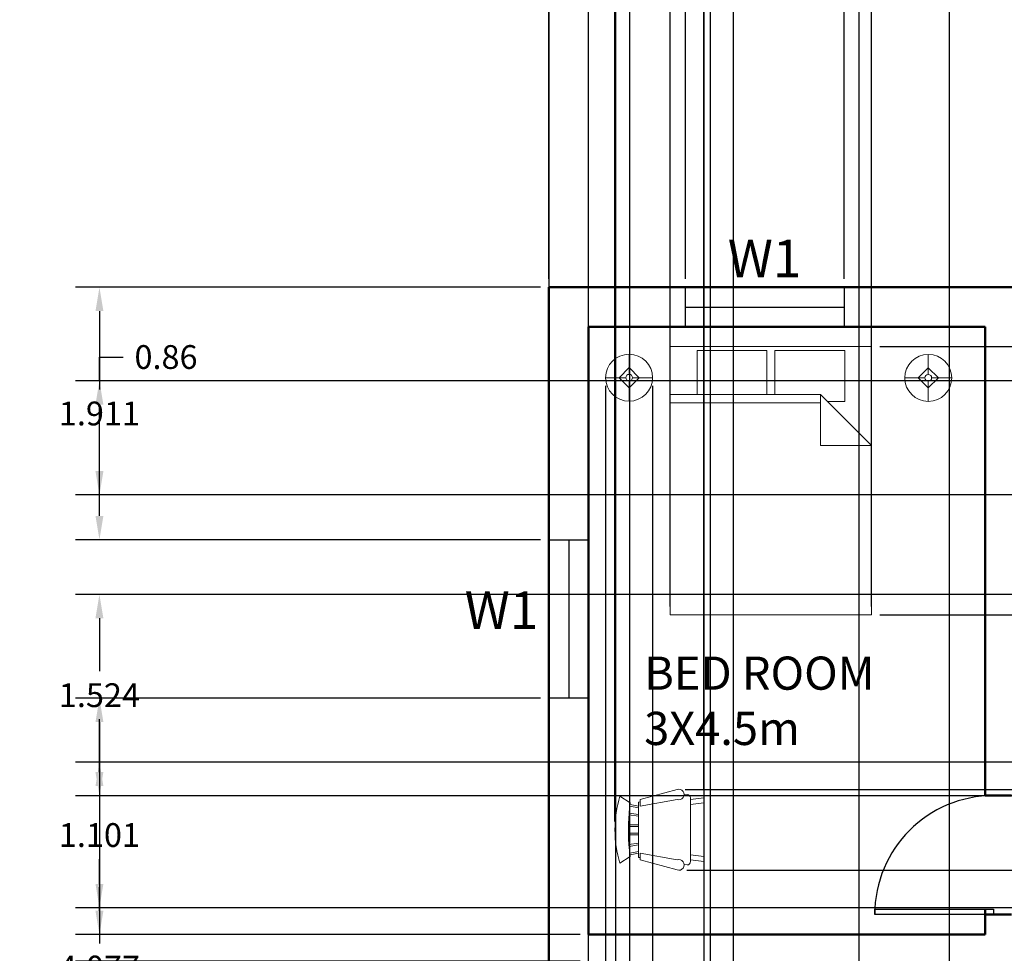
# Model space of a CAD drawing. Units: metres. Extents: x 2443.7 to 2482.9, y 2261.4 to 2287.
# Tile 3 of 8: x 2443.7 to 2451.1, y 2269.7 to 2276.8. Entities that reach past the tile are written whole.
import ezdxf

# ---------------------------------------------------------------- set-up
doc = ezdxf.new("R2010")
doc.units = ezdxf.units.M
for name, color, linetype, lineweight in [('A-ANNO-DIMS', 2, 'Continuous', 18), ('A-AREA-IDEN', 11, 'Continuous', 25), ('A-MODL', 7, 'Continuous', 25), ('A-WALL', 7, 'Continuous', 50), ('door', 6, 'Continuous', 25), ('furnitures', 20, 'Continuous', 18), ('text', 11, 'Continuous', 25), ('window', 3, 'Continuous', 25)]:
    doc.layers.add(name, color=color, linetype=linetype, lineweight=lineweight)
doc.styles.get("Standard").update_dxf_attribs({"font": 'arial.ttf'})
doc.dimstyles.get("Standard").update_dxf_attribs({"dimtxt": 0.18, "dimasz": 0.18, "dimexe": 0.18, "dimexo": 0.0625, "dimgap": 0.09, "dimtad": 0, "dimtih": 1, "dimtoh": 1, "dimdec": 4, "dimzin": 0, "dimdsep": 46, "dimtxsty": 'Standard', "dimcen": 0.09, "dimadec": 0, "dimazin": 0, "dimtfac": 1, "dimtdec": 4, "dimtofl": 0, "dimtmove": 0, "dimatfit": 3, "dimfxl": 1, "dimtolj": 1, "dimtzin": 0, "dimarcsym": 0})

# ---------------------------------------------------------------- blocks, each defined once
blk = doc.blocks.new('*U21')
for p, q in [((0, 0), (0, -6)), ((40, 0), (40, -6))]:
    blk.add_line(p, q)
blk.add_lwpolyline([(0, 0), (0, 40), (1.75, 40), (1.75, 0)], close=True)
blk.add_arc((0, 0), 40, 0, 90)
blk = doc.blocks.new('Bed - Queen')
for p, q in [((0, -80.00003), (0, 0)), ((0, 0), (59.99999, 0)), ((59.99999, 0), (59.99999, -80.00003)), ((7.99999, -1.2), (28.79998, -1.2)), ((7.99999, -14.4), (7.99999, -1.2)), ((28.79998, -1.2), (28.79998, -14.4)), ((31.19999, -1.2), (51.99999, -1.2)), ((31.19999, -14.4), (31.19999, -1.2)), ((51.99999, -1.2), (51.99999, -16.4)), ((0, -14.4), (44.8, -14.4)), ((59.99999, -29.6), (44.8, -14.4)), ((44.8, -14.4), (44.8, -29.6)), ((44.8, -16.8), (0, -16.8)), ((51.99999, -16.4), (46.79936, -16.4)), ((44.8, -29.6), (59.99999, -29.6)), ((59.99999, -80.00003), (0, -80.00003))]:
    blk.add_line(p, q)
blk = doc.blocks.new('Chair - Rocking')
for p, q in [((-8, -4.5), (-10, -1.5)), ((8, -4.5), (10, -1.5)), ((-7.5, -4.5), (-7, -7)), ((-6.5, -7), (-7.02225, -4.43)), ((-4.5, -7), (-4.96674, -4.19951)), ((-4, -7), (-4.40532, -4.16272)), ((-1.5, -4.05012), (-1.5, -7)), ((-1, -7), (-1, -4.05012)), ((1, -7), (1, -4.04655)), ((1.5, -4.05012), (1.5, -7)), ((4, -7), (4.40187, -4.18694)), ((4.5, -7), (4.96761, -4.19437)), ((6.5, -7), (7, -4.4057)), ((7.5, -4.5), (7, -7)), ((-9, -7.5), (-12, -18.49999)), ((-7, -7.5), (-9, -7.5)), ((-9, -18.49999), (-7, -7.5)), ((-8.23428, -6.99939), (-8.3093, -7.47958)), ((-8.23041, -7), (8.23915, -7)), ((7, -7.5), (9, -7.5)), ((9, -18.49999), (7, -7.5)), ((8.31071, -7.48854), (8.23449, -7.00073)), ((9, -7.5), (12, -18.49999)), ((-10.36644, -20.64523), (-10.5, -21.49999)), ((-9, -22.49999), (-9.5, -26.49999)), ((0, -22.49999), (-9.5, -22.49999)), ((-8, -26.49999), (-7.5, -22.49999)), ((0, -22.49999), (9.5, -22.49999)), ((8, -26.49999), (7.5, -22.49999)), ((9, -22.49999), (9.5, -26.49999)), ((10.5, -21.49999), (10.3575, -20.58798)), ((-9.5, -26.49999), (-8, -26.49999)), ((9.5, -26.49999), (8, -26.49999))]:
    blk.add_line(p, q)
for centre, radius, start, end in [((0, -34.08333), 34.08333, 72.93847, 107.0615), ((0, -68.25004), 64.25, 93.92211, 97.15267), ((0, -68.25004), 64.25, 82.84733, 93.92211), ((-10.5, -18.99999), 1.58114, 161.5651, 18.43495), ((10.5, -18.99999), 1.58114, 161.5651, 18.43495), ((-9.5, -21.49999), 1, 180, 270), ((9.5, -21.49999), 1, 270, 0)]:
    blk.add_arc(centre, radius, start, end)
blk = doc.blocks.new('Lamp - Table')
for p, q in [((0, 7), (0, 1)), ((0, 3), (-3, 0)), ((3, 0), (0, 3)), ((-1, 0), (-7, 0)), ((-3, 0), (0, -3)), ((0, -3), (3, 0)), ((1, 0), (7, 0)), ((0, -1), (0, -7))]:
    blk.add_line(p, q)
for radius in [7, 1]:
    blk.add_circle((0, 0), radius)
blk = doc.blocks.new('aditya')
at = {"layer": 'A-WALL'}
for p, q in [((0, 0), (0, 9.9)), ((0, 9.9), (10.2, 9.9)), ((0.3, 5), (0.3, 9.6)), ((0.3, 9.6), (3.3, 9.6)), ((3.3, 6.0498), (3.3, 9.6)), ((3.3, 5), (3.3, 5.1915)), ((0.3, 5), (3.3, 5))]:
    blk.add_line(p, q, dxfattribs=at)
for points in [[(3.3, 6.0498), (3.3, 6.0521), (3.5, 6.0521)], [(3.5, 5.1521), (3.3, 5.1521), (3.3, 5.1915)]]:
    blk.add_lwpolyline(points, dxfattribs=at)
at = {"layer": 'window'}
for p, q in [((1.0343, 9.75), (2.2343, 9.75)), ((0.15, 7.989), (0.15, 6.789))]:
    blk.add_line(p, q, dxfattribs=at)
for points in [[(1.0343, 9.6), (1.0343, 9.9), (2.2343, 9.9), (2.2343, 9.6)], [(0, 7.989), (0.3, 7.989), (0.3, 6.789), (0, 6.789)]]:
    blk.add_lwpolyline(points, close=True, dxfattribs=at)
at = {"layer": 'door', "xscale": 0.0224999999999983, "yscale": 0.0224999999999983, "zscale": 0.0224999999999983, "rotation": 90}
blk.add_blockref('*U21', (3.365, 5.1521), dxfattribs=at)
at = {"layer": 'furnitures', "xscale": 0.0254, "yscale": 0.0254, "zscale": 0.0254}
for name, p in [('Lamp - Table', (0.6073, 9.2154)), ('Bed - Queen', (0.9182, 9.4527)), ('Lamp - Table', (2.8707, 9.2141))]:
    blk.add_blockref(name, p, dxfattribs=at)
at = {"layer": 'furnitures', "xscale": 0.0254, "yscale": 0.0254, "zscale": 0.0254, "rotation": 90}
blk.add_blockref('Chair - Rocking', (0.5, 5.7938), dxfattribs=at)
at = {"layer": 'A-AREA-IDEN', "insert": (0.7212, 7.1044), "char_height": 0.250924, "attachment_point": 1}
blk.add_mtext_dynamic_manual_height_columns('{\\fArial|b1|i1|c0|p34;BED ROOM\\P3X4.5m}', width=10.569305, gutter_width=7.8414, heights=[0], dxfattribs=at)
at = {"layer": 'text'}
for p in [(1.3535, 9.9753), (-0.6369, 7.3126)]:
    blk.add_text('W1', height=0.28528, dxfattribs=at).set_placement(p)
blk = doc.blocks.new('*D26')
at = {"layer": 'A-ANNO-DIMS', "color": 0, "lineweight": -2, "transparency": 16777216}
for p, q in [((2447.6828, 2274.8222), (2447.6828, 2287.0152)), ((2448.7171, 2274.8222), (2448.7171, 2287.0152)), ((2447.5028, 2286.8352), (2447.3228, 2286.8352)), ((2448.8971, 2286.8352), (2449.0771, 2286.8352))]:
    blk.add_line(p, q, dxfattribs=at)
at = {"layer": 'A-ANNO-DIMS', "color": 0, "transparency": 16777216}
for points in [[(2447.5028, 2286.8652), (2447.5028, 2286.8052), (2447.6828, 2286.8352)], [(2448.8971, 2286.8652), (2448.8971, 2286.8052), (2448.7171, 2286.8352)]]:
    blk.add_solid(points, dxfattribs=at)
at = {"layer": 'Defpoints', "color": 0, "transparency": 16777216}
for p in [(2448.7171, 2286.8352), (2447.6828, 2274.7597), (2448.7171, 2274.7597)]:
    blk.add_point(p, dxfattribs=at)
at = {"layer": 'A-ANNO-DIMS', "color": 0, "transparency": 16777216, "insert": (2448.1999, 2286.8352), "char_height": 0.18, "attachment_point": 5}
blk.add_mtext('\\A1;1.03', dxfattribs=at)
blk = doc.blocks.new('*D27')
at = {"layer": 'A-ANNO-DIMS', "color": 0, "lineweight": -2, "transparency": 16777216}
for p, q in [((2448.7171, 2274.8222), (2448.7171, 2287.0152)), ((2449.9171, 2274.8222), (2449.9171, 2287.0152)), ((2448.8971, 2286.8352), (2449.0726, 2286.8352)), ((2449.7371, 2286.8352), (2449.5615, 2286.8352))]:
    blk.add_line(p, q, dxfattribs=at)
at = {"layer": 'A-ANNO-DIMS', "color": 0, "transparency": 16777216}
for points in [[(2448.8971, 2286.8652), (2448.8971, 2286.8052), (2448.7171, 2286.8352)], [(2449.7371, 2286.8652), (2449.7371, 2286.8052), (2449.9171, 2286.8352)]]:
    blk.add_solid(points, dxfattribs=at)
at = {"layer": 'Defpoints', "color": 0, "transparency": 16777216}
for p in [(2449.9171, 2286.8352), (2448.7171, 2274.7597), (2449.9171, 2274.7597)]:
    blk.add_point(p, dxfattribs=at)
at = {"layer": 'A-ANNO-DIMS', "color": 0, "transparency": 16777216, "insert": (2449.3171, 2286.8352), "char_height": 0.18, "attachment_point": 5}
blk.add_mtext('\\A1;1.2', dxfattribs=at)
blk = doc.blocks.new('*D28')
at = {"layer": 'A-ANNO-DIMS', "color": 0, "lineweight": -2, "transparency": 16777216}
for p, q in [((2449.9171, 2274.8222), (2449.9171, 2287.0152)), ((2451.4471, 2274.8222), (2451.4471, 2287.0152)), ((2450.0971, 2286.8352), (2450.3668, 2286.8352)), ((2451.2671, 2286.8352), (2450.9974, 2286.8352))]:
    blk.add_line(p, q, dxfattribs=at)
at = {"layer": 'A-ANNO-DIMS', "color": 0, "transparency": 16777216}
for points in [[(2450.0971, 2286.8652), (2450.0971, 2286.8052), (2449.9171, 2286.8352)], [(2451.2671, 2286.8652), (2451.2671, 2286.8052), (2451.4471, 2286.8352)]]:
    blk.add_solid(points, dxfattribs=at)
at = {"layer": 'Defpoints', "color": 0, "transparency": 16777216}
for p in [(2451.4471, 2286.8352), (2449.9171, 2274.7597), (2451.4471, 2274.7597)]:
    blk.add_point(p, dxfattribs=at)
at = {"layer": 'A-ANNO-DIMS', "color": 0, "transparency": 16777216, "insert": (2450.6821, 2286.8352), "char_height": 0.18, "attachment_point": 5}
blk.add_mtext('\\A1;1.53', dxfattribs=at)
blk = doc.blocks.new('*D32')
at = {"layer": 'A-ANNO-DIMS', "color": 0, "lineweight": -2, "transparency": 16777216}
for p, q in [((2447.6203, 2271.6487), (2444.1027, 2271.6487)), ((2444.2827, 2271.4687), (2444.2827, 2269.792)), ((2444.2827, 2267.7515), (2444.2827, 2269.4282)), ((2447.6203, 2267.5715), (2444.1027, 2267.5715))]:
    blk.add_line(p, q, dxfattribs=at)
at = {"layer": 'A-ANNO-DIMS', "color": 0, "transparency": 16777216}
for points in [[(2444.2527, 2271.4687), (2444.3127, 2271.4687), (2444.2827, 2271.6487)], [(2444.2527, 2267.7515), (2444.3127, 2267.7515), (2444.2827, 2267.5715)]]:
    blk.add_solid(points, dxfattribs=at)
at = {"layer": 'Defpoints', "color": 0, "transparency": 16777216}
for p in [(2444.2827, 2271.6487), (2447.6828, 2271.6487), (2447.6828, 2267.5715)]:
    blk.add_point(p, dxfattribs=at)
at = {"layer": 'A-ANNO-DIMS', "color": 0, "transparency": 16777216, "insert": (2444.2827, 2269.6101), "char_height": 0.18, "attachment_point": 5}
blk.add_mtext('\\A1;4.077', dxfattribs=at)
blk = doc.blocks.new('*D33')
at = {"layer": 'A-ANNO-DIMS', "color": 0, "lineweight": -2, "transparency": 16777216}
for p, q in [((2447.6203, 2274.7597), (2444.1027, 2274.7597)), ((2444.2827, 2274.5797), (2444.2827, 2273.9861)), ((2444.2827, 2273.0287), (2444.2827, 2273.6223)), ((2447.6203, 2272.8487), (2444.1027, 2272.8487))]:
    blk.add_line(p, q, dxfattribs=at)
at = {"layer": 'A-ANNO-DIMS', "color": 0, "transparency": 16777216}
for points in [[(2444.2527, 2274.5797), (2444.3127, 2274.5797), (2444.2827, 2274.7597)], [(2444.2527, 2273.0287), (2444.3127, 2273.0287), (2444.2827, 2272.8487)]]:
    blk.add_solid(points, dxfattribs=at)
at = {"layer": 'Defpoints', "color": 0, "transparency": 16777216}
for p in [(2444.2827, 2274.7597), (2447.6828, 2274.7597), (2447.6828, 2272.8487)]:
    blk.add_point(p, dxfattribs=at)
at = {"layer": 'A-ANNO-DIMS', "color": 0, "transparency": 16777216, "insert": (2444.2827, 2273.8042), "char_height": 0.18, "attachment_point": 5}
blk.add_mtext('\\A1;1.911', dxfattribs=at)
blk = doc.blocks.new('*D36')
at = {"layer": 'A-ANNO-DIMS', "color": 0, "lineweight": -2, "transparency": 16777216}
for p, q in [((2448.6009, 2272.3428), (2448.6009, 2287.0152)), ((2450.1249, 2272.3428), (2450.1249, 2287.0152)), ((2448.7809, 2286.8352), (2448.9781, 2286.8352)), ((2449.9449, 2286.8352), (2449.7478, 2286.8352))]:
    blk.add_line(p, q, dxfattribs=at)
at = {"layer": 'A-ANNO-DIMS', "color": 0, "transparency": 16777216}
for points in [[(2448.7809, 2286.8652), (2448.7809, 2286.8052), (2448.6009, 2286.8352)], [(2449.9449, 2286.8652), (2449.9449, 2286.8052), (2450.1249, 2286.8352)]]:
    blk.add_solid(points, dxfattribs=at)
at = {"layer": 'Defpoints', "color": 0, "transparency": 16777216}
for p in [(2450.1249, 2286.8352), (2448.6009, 2272.2803), (2450.1249, 2272.2803)]:
    blk.add_point(p, dxfattribs=at)
at = {"layer": 'A-ANNO-DIMS', "color": 0, "transparency": 16777216, "insert": (2449.3629, 2286.8352), "char_height": 0.18, "attachment_point": 5}
blk.add_mtext('\\A1;1.524', dxfattribs=at)
blk = doc.blocks.new('*D37')
at = {"layer": 'A-ANNO-DIMS', "color": 0, "lineweight": -2, "transparency": 16777216}
for p, q in [((2450.1874, 2274.3123), (2482.2428, 2274.3123)), ((2482.0628, 2274.1323), (2482.0628, 2273.4783)), ((2482.0628, 2272.4603), (2482.0628, 2273.1144)), ((2450.1874, 2272.2803), (2482.2428, 2272.2803))]:
    blk.add_line(p, q, dxfattribs=at)
at = {"layer": 'A-ANNO-DIMS', "color": 0, "transparency": 16777216}
for points in [[(2482.0328, 2274.1323), (2482.0928, 2274.1323), (2482.0628, 2274.3123)], [(2482.0328, 2272.4603), (2482.0928, 2272.4603), (2482.0628, 2272.2803)]]:
    blk.add_solid(points, dxfattribs=at)
at = {"layer": 'Defpoints', "color": 0, "transparency": 16777216}
for p in [(2450.1249, 2274.3123), (2482.0628, 2274.3123), (2450.1249, 2272.2803)]:
    blk.add_point(p, dxfattribs=at)
at = {"layer": 'A-ANNO-DIMS', "color": 0, "transparency": 16777216, "insert": (2482.0628, 2273.2963), "char_height": 0.18, "attachment_point": 5}
blk.add_mtext('\\A1;2.032', dxfattribs=at)
blk = doc.blocks.new('*D39')
at = {"layer": 'A-ANNO-DIMS', "color": 0, "lineweight": -2, "transparency": 16777216}
for p, q in [((2444.2827, 2274.0514), (2444.2827, 2274.2314)), ((2444.2827, 2274.2314), (2444.4627, 2274.2314)), ((2455.0752, 2274.0514), (2444.1027, 2274.0514)), ((2444.2827, 2273.3678), (2444.2827, 2273.8714)), ((2454.3132, 2273.1878), (2444.1027, 2273.1878))]:
    blk.add_line(p, q, dxfattribs=at)
at = {"layer": 'A-ANNO-DIMS', "color": 0, "transparency": 16777216}
for points in [[(2444.2527, 2273.8714), (2444.3127, 2273.8714), (2444.2827, 2274.0514)], [(2444.2527, 2273.3678), (2444.3127, 2273.3678), (2444.2827, 2273.1878)]]:
    blk.add_solid(points, dxfattribs=at)
at = {"layer": 'Defpoints', "color": 0, "transparency": 16777216}
for p in [(2444.2827, 2274.0514), (2455.1377, 2274.0514), (2454.3757, 2273.1878)]:
    blk.add_point(p, dxfattribs=at)
at = {"layer": 'A-ANNO-DIMS', "color": 0, "transparency": 16777216, "insert": (2444.7864, 2274.2314), "char_height": 0.18, "attachment_point": 5}
blk.add_mtext('\\A1;0.86', dxfattribs=at)
blk = doc.blocks.new('*D42')
at = {"layer": 'A-ANNO-DIMS', "color": 0, "lineweight": -2, "transparency": 16777216}
for p, q in [((2454.6838, 2272.434), (2444.1027, 2272.434)), ((2444.2827, 2272.254), (2444.2827, 2271.854)), ((2444.2827, 2271.09), (2444.2827, 2271.4901)), ((2454.6838, 2270.91), (2444.1027, 2270.91))]:
    blk.add_line(p, q, dxfattribs=at)
at = {"layer": 'A-ANNO-DIMS', "color": 0, "transparency": 16777216}
for points in [[(2444.2527, 2272.254), (2444.3127, 2272.254), (2444.2827, 2272.434)], [(2444.2527, 2271.09), (2444.3127, 2271.09), (2444.2827, 2270.91)]]:
    blk.add_solid(points, dxfattribs=at)
at = {"layer": 'Defpoints', "color": 0, "transparency": 16777216}
for p in [(2444.2827, 2272.434), (2454.7463, 2272.434), (2454.7463, 2270.91)]:
    blk.add_point(p, dxfattribs=at)
at = {"layer": 'A-ANNO-DIMS', "color": 0, "transparency": 16777216, "insert": (2444.2827, 2271.672), "char_height": 0.18, "attachment_point": 5}
blk.add_mtext('\\A1;1.524', dxfattribs=at)
blk = doc.blocks.new('*D45')
at = {"layer": 'A-ANNO-DIMS', "color": 0, "lineweight": -2, "transparency": 16777216}
for p, q in [((2452.0234, 2271.1636), (2444.1027, 2271.1636)), ((2444.2827, 2270.9836), (2444.2827, 2270.795)), ((2444.2827, 2270.2425), (2444.2827, 2270.4312)), ((2452.0234, 2270.0625), (2444.1027, 2270.0625))]:
    blk.add_line(p, q, dxfattribs=at)
at = {"layer": 'A-ANNO-DIMS', "color": 0, "transparency": 16777216}
for points in [[(2444.2527, 2270.9836), (2444.3127, 2270.9836), (2444.2827, 2271.1636)], [(2444.2527, 2270.2425), (2444.3127, 2270.2425), (2444.2827, 2270.0625)]]:
    blk.add_solid(points, dxfattribs=at)
at = {"layer": 'Defpoints', "color": 0, "transparency": 16777216}
for p in [(2444.2827, 2271.1636), (2452.0859, 2271.1636), (2452.0859, 2270.0625)]:
    blk.add_point(p, dxfattribs=at)
at = {"layer": 'A-ANNO-DIMS', "color": 0, "transparency": 16777216, "insert": (2444.2827, 2270.6131), "char_height": 0.18, "attachment_point": 5}
blk.add_mtext('\\A1;1.101', dxfattribs=at)
blk = doc.blocks.new('*D46')
at = {"layer": 'A-ANNO-DIMS', "color": 0, "lineweight": -2, "transparency": 16777216}
for p, q in [((2448.2963, 2267.4822), (2448.2963, 2287.0152)), ((2448.9059, 2267.4822), (2448.9059, 2287.0152)), ((2448.4763, 2286.8352), (2448.7259, 2286.8352)), ((2448.9059, 2286.8352), (2449.0859, 2286.8352))]:
    blk.add_line(p, q, dxfattribs=at)
at = {"layer": 'A-ANNO-DIMS', "color": 0, "transparency": 16777216}
for points in [[(2448.4763, 2286.8652), (2448.4763, 2286.8052), (2448.2963, 2286.8352)], [(2448.7259, 2286.8652), (2448.7259, 2286.8052), (2448.9059, 2286.8352)]]:
    blk.add_solid(points, dxfattribs=at)
at = {"layer": 'Defpoints', "color": 0, "transparency": 16777216}
for p in [(2448.9059, 2286.8352), (2448.2963, 2267.4197), (2448.9059, 2267.4197)]:
    blk.add_point(p, dxfattribs=at)
at = {"layer": 'A-ANNO-DIMS', "color": 0, "transparency": 16777216, "insert": (2449.3923, 2286.8352), "char_height": 0.18, "attachment_point": 5}
blk.add_mtext('\\A1;0.61', dxfattribs=at)
blk = doc.blocks.new('*D48')
at = {"layer": 'A-ANNO-DIMS', "color": 0, "lineweight": -2, "transparency": 16777216}
for p, q in [((2448.1904, 2269.4567), (2448.1904, 2287.0152)), ((2448.8583, 2269.4567), (2448.8583, 2287.0152)), ((2448.3704, 2286.8352), (2448.6783, 2286.8352)), ((2448.8583, 2286.8352), (2449.0383, 2286.8352))]:
    blk.add_line(p, q, dxfattribs=at)
at = {"layer": 'A-ANNO-DIMS', "color": 0, "transparency": 16777216}
for points in [[(2448.3704, 2286.8652), (2448.3704, 2286.8052), (2448.1904, 2286.8352)], [(2448.6783, 2286.8652), (2448.6783, 2286.8052), (2448.8583, 2286.8352)]]:
    blk.add_solid(points, dxfattribs=at)
at = {"layer": 'Defpoints', "color": 0, "transparency": 16777216}
for p in [(2448.8583, 2286.8352), (2448.1904, 2269.3942), (2448.8583, 2269.3942)]:
    blk.add_point(p, dxfattribs=at)
at = {"layer": 'A-ANNO-DIMS', "color": 0, "transparency": 16777216, "insert": (2449.4322, 2286.8352), "char_height": 0.18, "attachment_point": 5}
blk.add_mtext('\\A1;0.668', dxfattribs=at)
blk = doc.blocks.new('*D50')
at = {"layer": 'A-ANNO-DIMS', "color": 0, "lineweight": -2, "transparency": 16777216}
for p, q in [((2450.031, 2266.2523), (2450.031, 2287.0152)), ((2450.7143, 2266.2523), (2450.7143, 2287.0152)), ((2449.851, 2286.8352), (2449.671, 2286.8352)), ((2450.8943, 2286.8352), (2451.0743, 2286.8352))]:
    blk.add_line(p, q, dxfattribs=at)
at = {"layer": 'A-ANNO-DIMS', "color": 0, "transparency": 16777216}
for points in [[(2449.851, 2286.8652), (2449.851, 2286.8052), (2450.031, 2286.8352)], [(2450.8943, 2286.8652), (2450.8943, 2286.8052), (2450.7143, 2286.8352)]]:
    blk.add_solid(points, dxfattribs=at)
at = {"layer": 'Defpoints', "color": 0, "transparency": 16777216}
for p in [(2450.7143, 2286.8352), (2450.031, 2266.1898), (2450.7143, 2266.1898)]:
    blk.add_point(p, dxfattribs=at)
at = {"layer": 'A-ANNO-DIMS', "color": 0, "transparency": 16777216, "insert": (2450.3726, 2286.8352), "char_height": 0.18, "attachment_point": 5}
blk.add_mtext('\\A1;0.68', dxfattribs=at)
blk = doc.blocks.new('*D57')
at = {"layer": 'A-ANNO-DIMS', "color": 0, "lineweight": -2, "transparency": 16777216}
for p, q in [((2448.1827, 2270.716), (2448.1827, 2287.0152)), ((2448.8558, 2270.9573), (2448.8558, 2287.0152)), ((2448.3627, 2286.8352), (2448.6758, 2286.8352)), ((2448.8558, 2286.8352), (2449.0358, 2286.8352))]:
    blk.add_line(p, q, dxfattribs=at)
at = {"layer": 'A-ANNO-DIMS', "color": 0, "transparency": 16777216}
for points in [[(2448.3627, 2286.8652), (2448.3627, 2286.8052), (2448.1827, 2286.8352)], [(2448.6758, 2286.8652), (2448.6758, 2286.8052), (2448.8558, 2286.8352)]]:
    blk.add_solid(points, dxfattribs=at)
at = {"layer": 'Defpoints', "color": 0, "transparency": 16777216}
for p in [(2448.8558, 2286.8352), (2448.8558, 2270.8948), (2448.1827, 2270.6535)]:
    blk.add_point(p, dxfattribs=at)
at = {"layer": 'A-ANNO-DIMS', "color": 0, "transparency": 16777216, "insert": (2449.4295, 2286.8352), "char_height": 0.18, "attachment_point": 5}
blk.add_mtext('\\A1;0.673', dxfattribs=at)
blk = doc.blocks.new('*D58')
at = {"layer": 'A-ANNO-DIMS', "color": 0, "lineweight": -2, "transparency": 16777216}
for p, q in [((2448.7151, 2270.9583), (2482.2428, 2270.9583)), ((2482.0628, 2270.7783), (2482.0628, 2270.5266)), ((2448.7277, 2270.3466), (2482.2428, 2270.3466)), ((2482.0628, 2270.3466), (2482.0628, 2270.1666)), ((2482.0628, 2270.1666), (2481.8828, 2270.1666))]:
    blk.add_line(p, q, dxfattribs=at)
at = {"layer": 'A-ANNO-DIMS', "color": 0, "transparency": 16777216}
for points in [[(2482.0328, 2270.7783), (2482.0928, 2270.7783), (2482.0628, 2270.9583)], [(2482.0328, 2270.5266), (2482.0928, 2270.5266), (2482.0628, 2270.3466)]]:
    blk.add_solid(points, dxfattribs=at)
at = {"layer": 'Defpoints', "color": 0, "transparency": 16777216}
for p in [(2448.6526, 2270.9583), (2448.6652, 2270.3466), (2482.0628, 2270.3466)]:
    blk.add_point(p, dxfattribs=at)
at = {"layer": 'A-ANNO-DIMS', "color": 0, "transparency": 16777216, "insert": (2481.5764, 2270.1666), "char_height": 0.18, "attachment_point": 5}
blk.add_mtext('\\A1;0.61', dxfattribs=at)
blk = doc.blocks.new('*D59')
at = {"layer": 'A-ANNO-DIMS', "color": 0, "lineweight": -2, "transparency": 16777216}
for p, q in [((2448.1123, 2274.0125), (2448.1123, 2261.3876)), ((2448.4679, 2274.0125), (2448.4679, 2261.3876)), ((2447.9323, 2261.5676), (2447.7523, 2261.5676)), ((2448.6479, 2261.5676), (2448.8279, 2261.5676))]:
    blk.add_line(p, q, dxfattribs=at)
at = {"layer": 'A-ANNO-DIMS', "color": 0, "transparency": 16777216}
for points in [[(2447.9323, 2261.5976), (2447.9323, 2261.5376), (2448.1123, 2261.5676)], [(2448.6479, 2261.5976), (2448.6479, 2261.5376), (2448.4679, 2261.5676)]]:
    blk.add_solid(points, dxfattribs=at)
at = {"layer": 'Defpoints', "color": 0, "transparency": 16777216}
for p in [(2448.1123, 2274.075), (2448.4679, 2274.075), (2448.4679, 2261.5676)]:
    blk.add_point(p, dxfattribs=at)
at = {"layer": 'A-ANNO-DIMS', "color": 0, "transparency": 16777216, "insert": (2449.1516, 2261.5676), "char_height": 0.18, "attachment_point": 5}
blk.add_mtext('\\A1;0.36', dxfattribs=at)
blk = doc.blocks.new('*D61')
at = {"layer": 'A-ANNO-DIMS', "color": 0, "lineweight": -2, "transparency": 16777216}
for p, q in [((2444.2827, 2270.0397), (2444.2827, 2270.2197)), ((2447.9203, 2269.8597), (2444.1027, 2269.8597)), ((2447.9203, 2269.6597), (2444.1027, 2269.6597)), ((2444.2827, 2269.4797), (2444.2827, 2269.2997)), ((2444.2827, 2269.2997), (2444.1027, 2269.2997))]:
    blk.add_line(p, q, dxfattribs=at)
at = {"layer": 'A-ANNO-DIMS', "color": 0, "transparency": 16777216}
for points in [[(2444.2527, 2270.0397), (2444.3127, 2270.0397), (2444.2827, 2269.8597)], [(2444.2527, 2269.4797), (2444.3127, 2269.4797), (2444.2827, 2269.6597)]]:
    blk.add_solid(points, dxfattribs=at)
at = {"layer": 'Defpoints', "color": 0, "transparency": 16777216}
for p in [(2447.9828, 2269.8597), (2444.2827, 2269.6597), (2447.9828, 2269.6597)]:
    blk.add_point(p, dxfattribs=at)
at = {"layer": 'A-ANNO-DIMS', "color": 0, "transparency": 16777216, "insert": (2443.8498, 2269.2997), "char_height": 0.18, "attachment_point": 5}
blk.add_mtext('\\A1;0.2', dxfattribs=at)
blk = doc.blocks.new('*D62')
at = {"layer": 'A-ANNO-DIMS', "color": 0, "lineweight": -2, "transparency": 16777216}
for p, q in [((2447.982762, 2265.222173), (2447.982762, 2287.015188)), ((2449.080462, 2266.304727), (2449.080462, 2287.015188)), ((2447.802762, 2286.835188), (2447.622762, 2286.835188)), ((2449.260462, 2286.835188), (2449.440462, 2286.835188))]:
    blk.add_line(p, q, dxfattribs=at)
at = {"layer": 'A-ANNO-DIMS', "color": 0, "transparency": 16777216}
for points in [[(2447.802762, 2286.865188), (2447.802762, 2286.805188), (2447.982762, 2286.835188)], [(2449.260462, 2286.865188), (2449.260462, 2286.805188), (2449.080462, 2286.835188)]]:
    blk.add_solid(points, dxfattribs=at)
at = {"layer": 'Defpoints', "color": 0, "transparency": 16777216}
for p in [(2449.080462, 2286.835188), (2449.080462, 2266.242227), (2447.982762, 2265.159673)]:
    blk.add_point(p, dxfattribs=at)
at = {"layer": 'A-ANNO-DIMS', "color": 0, "transparency": 16777216, "insert": (2448.531612, 2286.835188), "char_height": 0.18, "attachment_point": 5}
blk.add_mtext('\\A1;1.10', dxfattribs=at)
blk = doc.blocks.new('*D63')
at = {"layer": 'A-ANNO-DIMS', "color": 0, "lineweight": -2, "transparency": 16777216}
for p, q in [((2447.6828, 2278.9987), (2447.6828, 2261.3876)), ((2457.8828, 2278.9987), (2457.8828, 2261.3876)), ((2447.8628, 2261.5676), (2452.4684, 2261.5676)), ((2457.7028, 2261.5676), (2453.0971, 2261.5676))]:
    blk.add_line(p, q, dxfattribs=at)
at = {"layer": 'A-ANNO-DIMS', "color": 0, "transparency": 16777216}
for points in [[(2447.8628, 2261.5976), (2447.8628, 2261.5376), (2447.6828, 2261.5676)], [(2457.7028, 2261.5976), (2457.7028, 2261.5376), (2457.8828, 2261.5676)]]:
    blk.add_solid(points, dxfattribs=at)
at = {"layer": 'Defpoints', "color": 0, "transparency": 16777216}
for p in [(2447.6828, 2279.0612), (2457.8828, 2279.0612), (2457.8828, 2261.5676)]:
    blk.add_point(p, dxfattribs=at)
at = {"layer": 'A-ANNO-DIMS', "color": 0, "transparency": 16777216, "insert": (2452.7828, 2261.5676), "char_height": 0.18, "attachment_point": 5}
blk.add_mtext('\\A1;10.2', dxfattribs=at)

msp = doc.modelspace()

# ---------------------------------------------------------------- block references
at = {"layer": 'A-MODL'}
msp.add_blockref('aditya', (2447.682762, 2264.859673), dxfattribs=at)

# ---------------------------------------------------------------- dimensions: what is measured, and where the dimension line sits
at = {"layer": 'A-ANNO-DIMS'}
for base, p1, p2, override, picture, middle in [((2448.717083, 2286.835188), (2447.682762, 2274.759673), (2448.717083, 2274.759673), {"dimdec": 2, "dimlfac": 1, "dimrnd": 0, "dimzin": 0, "dimdsep": 46, "dimlunit": 2}, '*D26', (2448.199922, 2286.835188)), ((2449.080462, 2286.835188), (2447.982762, 2265.159673), (2449.080462, 2266.242227), {"dimdec": 2, "dimlfac": 1, "dimrnd": 0, "dimzin": 0, "dimdsep": 46, "dimlunit": 2}, '*D62', (2448.531612, 2286.835188)), ((2448.855842, 2286.835188), (2448.182742, 2270.653501), (2448.855842, 2270.894801), {"dimdec": 3, "dimlfac": 1, "dimrnd": 0, "dimzin": 0, "dimdsep": 46, "dimlunit": 2}, '*D57', (2449.429546, 2286.835188)), ((2448.858297, 2286.835188), (2448.190396, 2269.394205), (2448.858297, 2269.394205), {"dimdec": 3, "dimlfac": 1, "dimrnd": 0, "dimzin": 0, "dimdsep": 46, "dimlunit": 2}, '*D48', (2449.432185, 2286.835188)), ((2448.905882, 2286.835188), (2448.296282, 2267.419676), (2448.905882, 2267.419676), {"dimdec": 2, "dimlfac": 1, "dimrnd": 0, "dimzin": 0, "dimdsep": 46, "dimlunit": 2}, '*D46', (2449.392287, 2286.835188)), ((2450.124936, 2286.835188), (2448.600936, 2272.280339), (2450.124936, 2272.280339), {"dimdec": 3, "dimlfac": 1, "dimrnd": 0, "dimzin": 0, "dimdsep": 46, "dimlunit": 2}, '*D36', (2449.362936, 2286.835188)), ((2449.917083, 2286.835188), (2448.717083, 2274.759673), (2449.917083, 2274.759673), {"dimdec": 1, "dimlfac": 1, "dimrnd": 0, "dimzin": 0, "dimdsep": 46, "dimlunit": 2}, '*D27', (2449.317083, 2286.835188)), ((2450.714284, 2286.835188), (2450.030991, 2266.189812), (2450.714284, 2266.189812), {"dimdec": 2, "dimlfac": 1, "dimrnd": 0, "dimzin": 0, "dimdsep": 46, "dimlunit": 2}, '*D50', (2450.372638, 2286.835188)), ((2451.44713, 2286.835188), (2449.917083, 2274.759673), (2451.44713, 2274.759673), {"dimdec": 2, "dimlfac": 1, "dimrnd": 0, "dimzin": 0, "dimdsep": 46, "dimlunit": 2}, '*D28', (2450.682106, 2286.835188)), ((2457.882762, 2261.567605), (2447.682762, 2279.061188), (2457.882762, 2279.061188), {"dimdec": 1, "dimlfac": 1, "dimrnd": 0, "dimzin": 0, "dimdsep": 46, "dimlunit": 2}, '*D63', (2452.782762, 2261.567605)), ((2448.467902, 2261.567605), (2448.112302, 2274.07505), (2448.467902, 2274.07505), {"dimdec": 2, "dimlfac": 1, "dimrnd": 0, "dimzin": 0, "dimdsep": 46, "dimlunit": 2}, '*D59', (2449.15162, 2261.567605))]:
    dim = msp.add_linear_dim(base=base, p1=p1, p2=p2, dimstyle='Standard', override=override, dxfattribs=at)
    dim.commit()
    dim.dimension.update_dxf_attribs({"geometry": picture, "text_midpoint": middle})
for base, p1, p2, override, picture, middle in [((2444.282724, 2274.759673), (2447.682762, 2272.848723), (2447.682762, 2274.759673), {"dimdec": 3, "dimlfac": 1, "dimrnd": 0, "dimzin": 0, "dimdsep": 46, "dimlunit": 2}, '*D33', (2444.282724, 2273.804198)), ((2444.282724, 2274.051415), (2454.375659, 2273.187816), (2455.13766, 2274.051415), {"dimdec": 2, "dimlfac": 1, "dimrnd": 0, "dimzin": 0, "dimdsep": 46, "dimlunit": 2}, '*D39', (2444.786442, 2274.231415)), ((2482.062768, 2274.312339), (2450.124936, 2272.280339), (2450.124936, 2274.312339), {"dimdec": 3, "dimlfac": 1, "dimrnd": 0, "dimzin": 0, "dimdsep": 46, "dimlunit": 2}, '*D37', (2482.062768, 2273.296339)), ((2444.282724, 2272.434047), (2454.746253, 2270.910047), (2454.746253, 2272.434047), {"dimdec": 3, "dimlfac": 1, "dimrnd": 0, "dimzin": 0, "dimdsep": 46, "dimlunit": 2}, '*D42', (2444.282724, 2271.672047)), ((2444.282724, 2271.648723), (2447.682762, 2267.571466), (2447.682762, 2271.648723), {"dimdec": 3, "dimlfac": 1, "dimrnd": 0, "dimzin": 0, "dimdsep": 46, "dimlunit": 2}, '*D32', (2444.282724, 2269.610094)), ((2444.282724, 2271.163582), (2452.085916, 2270.062544), (2452.085916, 2271.163582), {"dimdec": 3, "dimlfac": 1, "dimrnd": 0, "dimzin": 0, "dimdsep": 46, "dimlunit": 2}, '*D45', (2444.282724, 2270.613063)), ((2482.062768, 2270.346637), (2448.652642, 2270.958301), (2448.665238, 2270.346637), {"dimdec": 2, "dimlfac": 1, "dimrnd": 0, "dimzin": 0, "dimdsep": 46, "dimlunit": 2}, '*D58', (2481.576363, 2270.166637)), ((2444.282724, 2269.659673), (2447.982762, 2269.859673), (2447.982762, 2269.659673), {"dimdec": 1, "dimlfac": 1, "dimrnd": 0, "dimzin": 0, "dimdsep": 46, "dimlunit": 2}, '*D61', (2443.849791, 2269.299673))]:
    dim = msp.add_linear_dim(base=base, p1=p1, p2=p2, angle=90, dimstyle='Standard', override=override, dxfattribs=at)
    dim.commit()
    dim.dimension.update_dxf_attribs({"geometry": picture, "text_midpoint": middle})

doc.saveas('drawing.dxf')
